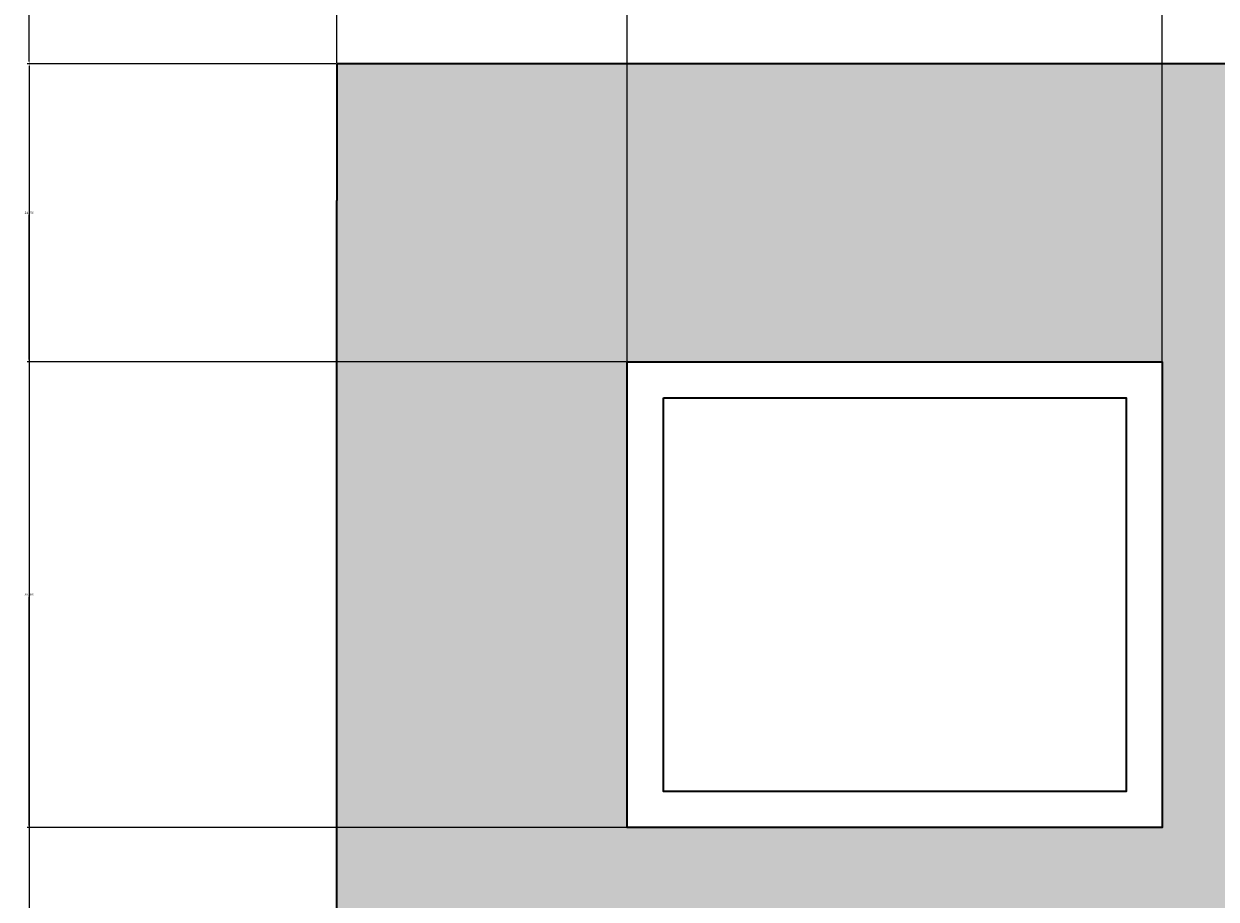
# Model space of a CAD drawing. Units: inches. Extents: x 93 to 565, y 123 to 656.
# Tile 6 of 18: x 93 to 192, y 450 to 522. Entities that reach past the tile are written whole.
import ezdxf

# ---------------------------------------------------------------- set-up
doc = ezdxf.new("R2010")
doc.units = ezdxf.units.IN
doc.header["$MEASUREMENT"] = 0
for name, color, linetype, lineweight in [('A-ANNO-DIMS', 2, 'Continuous', 18), ('A-ELEV', 7, 'Continuous', 35), ('A-WALL-PATT', 8, 'Continuous', 13)]:
    doc.layers.add(name, color=color, linetype=linetype, lineweight=lineweight)
doc.styles.get("Standard").update_dxf_attribs({"font": 'arial.ttf'})
doc.dimstyles.get("Standard").update_dxf_attribs({"dimtxt": 0.18, "dimasz": 0.18, "dimexe": 0.18, "dimexo": 0.0625, "dimgap": 0.09, "dimtad": 0, "dimtih": 1, "dimtoh": 1, "dimdec": 4, "dimzin": 0, "dimdsep": 46, "dimtxsty": 'Standard', "dimcen": 0.09, "dimadec": 0, "dimazin": 0, "dimtfac": 1, "dimtdec": 4, "dimtofl": 0, "dimtmove": 0, "dimatfit": 3, "dimfxl": 1, "dimtolj": 1, "dimtzin": 0, "dimarcsym": 0})

# ---------------------------------------------------------------- blocks, each defined once
blk = doc.blocks.new('*D26')
at = {"layer": 'A-ANNO-DIMS', "color": 0, "lineweight": -2, "transparency": 16777216}
for p, q in [((119.079, 519.162), (119.079, 656.135)), ((119.259, 655.955), (328.787, 655.955)), ((538.899, 655.955), (329.372, 655.955)), ((539.079, 630.467), (539.079, 656.135))]:
    blk.add_line(p, q, dxfattribs=at)
at = {"layer": 'A-ANNO-DIMS', "color": 0, "transparency": 16777216}
for points in [[(119.259, 655.985), (119.259, 655.925), (119.079, 655.955)], [(538.899, 655.985), (538.899, 655.925), (539.079, 655.955)]]:
    blk.add_solid(points, dxfattribs=at)
at = {"layer": 'Defpoints', "color": 0, "transparency": 16777216}
for p in [(539.079, 655.955), (539.079, 630.405), (119.079, 519.1)]:
    blk.add_point(p, dxfattribs=at)
at = {"layer": 'A-ANNO-DIMS', "color": 0, "transparency": 16777216, "insert": (329.079, 655.955), "char_height": 0.18, "attachment_point": 5}
blk.add_mtext('\\A1;420', dxfattribs=at)
blk = doc.blocks.new('*D27')
at = {"layer": 'A-ANNO-DIMS', "color": 0, "lineweight": -2, "transparency": 16777216}
for p, q in [((210.544, 519.037), (210.544, 134.002)), ((119.079, 159.67), (119.079, 134.002)), ((119.259, 134.182), (164.418, 134.182)), ((210.364, 134.182), (165.205, 134.182))]:
    blk.add_line(p, q, dxfattribs=at)
at = {"layer": 'A-ANNO-DIMS', "color": 0, "transparency": 16777216}
for points in [[(119.259, 134.212), (119.259, 134.152), (119.079, 134.182)], [(210.364, 134.212), (210.364, 134.152), (210.544, 134.182)]]:
    blk.add_solid(points, dxfattribs=at)
at = {"layer": 'Defpoints', "color": 0, "transparency": 16777216}
for p in [(210.544, 519.1), (119.079, 159.732), (210.544, 134.182)]:
    blk.add_point(p, dxfattribs=at)
at = {"layer": 'A-ANNO-DIMS', "color": 0, "transparency": 16777216, "insert": (164.812, 134.182), "char_height": 0.18, "attachment_point": 5}
blk.add_mtext('\\A1;91.46', dxfattribs=at)
blk = doc.blocks.new('*D31')
at = {"layer": 'A-ANNO-DIMS', "color": 0, "lineweight": -2, "transparency": 16777216}
for p, q in [((417.872, 630.405), (564.809, 630.405)), ((564.629, 630.225), (564.629, 395.25)), ((564.629, 159.912), (564.629, 394.887)), ((119.142, 159.732), (564.809, 159.732))]:
    blk.add_line(p, q, dxfattribs=at)
at = {"layer": 'A-ANNO-DIMS', "color": 0, "transparency": 16777216}
for points in [[(564.599, 630.225), (564.659, 630.225), (564.629, 630.405)], [(564.599, 159.912), (564.659, 159.912), (564.629, 159.732)]]:
    blk.add_solid(points, dxfattribs=at)
at = {"layer": 'Defpoints', "color": 0, "transparency": 16777216}
for p in [(417.81, 630.405), (564.629, 630.405), (119.079, 159.732)]:
    blk.add_point(p, dxfattribs=at)
at = {"layer": 'A-ANNO-DIMS', "color": 0, "transparency": 16777216, "insert": (564.629, 395.069), "char_height": 0.18, "attachment_point": 5}
blk.add_mtext('\\A1;470.7', dxfattribs=at)
blk = doc.blocks.new('*D35')
at = {"layer": 'A-ANNO-DIMS', "color": 0, "lineweight": -2, "transparency": 16777216}
for p, q in [((119.017, 519.1), (93.349, 519.1)), ((93.529, 518.92), (93.529, 441.598)), ((93.529, 363.912), (93.529, 441.234)), ((286.625, 363.732), (93.349, 363.732))]:
    blk.add_line(p, q, dxfattribs=at)
at = {"layer": 'A-ANNO-DIMS', "color": 0, "transparency": 16777216}
for points in [[(93.499, 518.92), (93.559, 518.92), (93.529, 519.1)], [(93.499, 363.912), (93.559, 363.912), (93.529, 363.732)]]:
    blk.add_solid(points, dxfattribs=at)
at = {"layer": 'Defpoints', "color": 0, "transparency": 16777216}
for p in [(93.529, 519.1), (119.079, 519.1), (286.687, 363.732)]:
    blk.add_point(p, dxfattribs=at)
at = {"layer": 'A-ANNO-DIMS', "color": 0, "transparency": 16777216, "insert": (93.529, 441.416), "char_height": 0.18, "attachment_point": 5}
blk.add_mtext('\\A1;155.37', dxfattribs=at)
blk = doc.blocks.new('*D36')
at = {"layer": 'A-ANNO-DIMS', "color": 0, "lineweight": -2, "transparency": 16777216}
for p, q in [((417.747, 594.405), (93.349, 594.405)), ((93.529, 594.225), (93.529, 556.934)), ((93.529, 519.28), (93.529, 556.57)), ((119.017, 519.1), (93.349, 519.1))]:
    blk.add_line(p, q, dxfattribs=at)
at = {"layer": 'A-ANNO-DIMS', "color": 0, "transparency": 16777216}
for points in [[(93.499, 594.225), (93.559, 594.225), (93.529, 594.405)], [(93.499, 519.28), (93.559, 519.28), (93.529, 519.1)]]:
    blk.add_solid(points, dxfattribs=at)
at = {"layer": 'Defpoints', "color": 0, "transparency": 16777216}
for p in [(93.529, 594.405), (417.81, 594.405), (119.079, 519.1)]:
    blk.add_point(p, dxfattribs=at)
at = {"layer": 'A-ANNO-DIMS', "color": 0, "transparency": 16777216, "insert": (93.529, 556.752), "char_height": 0.18, "attachment_point": 5}
blk.add_mtext('\\A1;75.3', dxfattribs=at)
blk = doc.blocks.new('*D46')
at = {"layer": 'A-ANNO-DIMS', "color": 0, "lineweight": -2, "transparency": 16777216}
for p, q in [((143.149, 455.658), (93.349, 455.658)), ((93.529, 455.478), (93.529, 443.086)), ((93.529, 430.331), (93.529, 442.722)), ((143.149, 430.151), (93.349, 430.151))]:
    blk.add_line(p, q, dxfattribs=at)
at = {"layer": 'A-ANNO-DIMS', "color": 0, "transparency": 16777216}
for points in [[(93.499, 455.478), (93.559, 455.478), (93.529, 455.658)], [(93.499, 430.331), (93.559, 430.331), (93.529, 430.151)]]:
    blk.add_solid(points, dxfattribs=at)
at = {"layer": 'Defpoints', "color": 0, "transparency": 16777216}
for p in [(93.529, 455.658), (143.212, 455.658), (143.212, 430.151)]:
    blk.add_point(p, dxfattribs=at)
at = {"layer": 'A-ANNO-DIMS', "color": 0, "transparency": 16777216, "insert": (93.529, 442.904), "char_height": 0.18, "attachment_point": 5}
blk.add_mtext('\\A1;25.507', dxfattribs=at)
blk = doc.blocks.new('*D47')
at = {"layer": 'A-ANNO-DIMS', "color": 0, "lineweight": -2, "transparency": 16777216}
for p, q in [((143.149, 494.343), (93.349, 494.343)), ((93.529, 494.163), (93.529, 475.183)), ((93.529, 455.838), (93.529, 474.819)), ((143.149, 455.658), (93.349, 455.658))]:
    blk.add_line(p, q, dxfattribs=at)
at = {"layer": 'A-ANNO-DIMS', "color": 0, "transparency": 16777216}
for points in [[(93.499, 494.163), (93.559, 494.163), (93.529, 494.343)], [(93.499, 455.838), (93.559, 455.838), (93.529, 455.658)]]:
    blk.add_solid(points, dxfattribs=at)
at = {"layer": 'Defpoints', "color": 0, "transparency": 16777216}
for p in [(93.529, 494.343), (143.212, 494.343), (143.212, 455.658)]:
    blk.add_point(p, dxfattribs=at)
at = {"layer": 'A-ANNO-DIMS', "color": 0, "transparency": 16777216, "insert": (93.529, 475.001), "char_height": 0.18, "attachment_point": 5}
blk.add_mtext('\\A1;38.685', dxfattribs=at)
blk = doc.blocks.new('*D48')
at = {"layer": 'A-ANNO-DIMS', "color": 0, "lineweight": -2, "transparency": 16777216}
for p, q in [((119.017, 519.1), (93.349, 519.1)), ((93.529, 518.92), (93.529, 506.904)), ((93.529, 494.523), (93.529, 506.54)), ((143.149, 494.343), (93.349, 494.343))]:
    blk.add_line(p, q, dxfattribs=at)
at = {"layer": 'A-ANNO-DIMS', "color": 0, "transparency": 16777216}
for points in [[(93.499, 518.92), (93.559, 518.92), (93.529, 519.1)], [(93.499, 494.523), (93.559, 494.523), (93.529, 494.343)]]:
    blk.add_solid(points, dxfattribs=at)
at = {"layer": 'Defpoints', "color": 0, "transparency": 16777216}
for p in [(93.529, 519.1), (119.079, 519.1), (143.212, 494.343)]:
    blk.add_point(p, dxfattribs=at)
at = {"layer": 'A-ANNO-DIMS', "color": 0, "transparency": 16777216, "insert": (93.529, 506.722), "char_height": 0.18, "attachment_point": 5}
blk.add_mtext('\\A1;24.756', dxfattribs=at)
blk = doc.blocks.new('*D49')
at = {"layer": 'A-ANNO-DIMS', "color": 0, "lineweight": -2, "transparency": 16777216}
for p, q in [((119.079, 519.162), (119.079, 656.135)), ((119.259, 655.955), (130.75, 655.955)), ((143.032, 655.955), (131.541, 655.955)), ((143.212, 494.406), (143.212, 656.135))]:
    blk.add_line(p, q, dxfattribs=at)
at = {"layer": 'A-ANNO-DIMS', "color": 0, "transparency": 16777216}
for points in [[(119.259, 655.985), (119.259, 655.925), (119.079, 655.955)], [(143.032, 655.985), (143.032, 655.925), (143.212, 655.955)]]:
    blk.add_solid(points, dxfattribs=at)
at = {"layer": 'Defpoints', "color": 0, "transparency": 16777216}
for p in [(143.212, 655.955), (119.079, 519.1), (143.212, 494.343)]:
    blk.add_point(p, dxfattribs=at)
at = {"layer": 'A-ANNO-DIMS', "color": 0, "transparency": 16777216, "insert": (131.146, 655.955), "char_height": 0.18, "attachment_point": 5}
blk.add_mtext('\\A1;24.13', dxfattribs=at)
blk = doc.blocks.new('*D50')
at = {"layer": 'A-ANNO-DIMS', "color": 0, "lineweight": -2, "transparency": 16777216}
for p, q in [((143.212, 494.406), (143.212, 656.135)), ((143.392, 655.955), (165.033, 655.955)), ((187.468, 655.955), (165.827, 655.955)), ((187.648, 494.406), (187.648, 656.135))]:
    blk.add_line(p, q, dxfattribs=at)
at = {"layer": 'A-ANNO-DIMS', "color": 0, "transparency": 16777216}
for points in [[(143.392, 655.985), (143.392, 655.925), (143.212, 655.955)], [(187.468, 655.985), (187.468, 655.925), (187.648, 655.955)]]:
    blk.add_solid(points, dxfattribs=at)
at = {"layer": 'Defpoints', "color": 0, "transparency": 16777216}
for p in [(187.648, 655.955), (143.212, 494.343), (187.648, 494.343)]:
    blk.add_point(p, dxfattribs=at)
at = {"layer": 'A-ANNO-DIMS', "color": 0, "transparency": 16777216, "insert": (165.43, 655.955), "char_height": 0.18, "attachment_point": 5}
blk.add_mtext('\\A1;44.44', dxfattribs=at)
blk = doc.blocks.new('*D105')
at = {"layer": 'A-ANNO-DIMS', "color": 0, "lineweight": -2, "transparency": 16777216}
for p, q in [((119.079, 519.162), (119.079, 656.135)), ((119.259, 655.955), (328.542, 655.955)), ((538.899, 655.955), (329.616, 655.955)), ((539.079, 630.467), (539.079, 656.135))]:
    blk.add_line(p, q, dxfattribs=at)
at = {"layer": 'A-ANNO-DIMS', "color": 0, "transparency": 16777216}
for points in [[(119.259, 655.985), (119.259, 655.925), (119.079, 655.955)], [(538.899, 655.985), (538.899, 655.925), (539.079, 655.955)]]:
    blk.add_solid(points, dxfattribs=at)
at = {"layer": 'Defpoints', "color": 0, "transparency": 16777216}
for p in [(539.079, 655.955), (539.079, 630.405), (119.079, 519.1)]:
    blk.add_point(p, dxfattribs=at)
at = {"layer": 'A-ANNO-DIMS', "color": 0, "transparency": 16777216, "insert": (329.079, 655.955), "char_height": 0.18, "attachment_point": 5}
blk.add_mtext('\\A1;420.000', dxfattribs=at)
blk = doc.blocks.new('*D106')
at = {"layer": 'A-ANNO-DIMS', "color": 0, "lineweight": -2, "transparency": 16777216}
for p, q in [((210.544, 519.037), (210.544, 134.002)), ((119.079, 159.67), (119.079, 134.002)), ((119.259, 134.182), (164.348, 134.182)), ((210.364, 134.182), (165.276, 134.182))]:
    blk.add_line(p, q, dxfattribs=at)
at = {"layer": 'A-ANNO-DIMS', "color": 0, "transparency": 16777216}
for points in [[(119.259, 134.212), (119.259, 134.152), (119.079, 134.182)], [(210.364, 134.212), (210.364, 134.152), (210.544, 134.182)]]:
    blk.add_solid(points, dxfattribs=at)
at = {"layer": 'Defpoints', "color": 0, "transparency": 16777216}
for p in [(210.544, 519.1), (119.079, 159.732), (210.544, 134.182)]:
    blk.add_point(p, dxfattribs=at)
at = {"layer": 'A-ANNO-DIMS', "color": 0, "transparency": 16777216, "insert": (164.812, 134.182), "char_height": 0.18, "attachment_point": 5}
blk.add_mtext('\\A1;91.465', dxfattribs=at)
blk = doc.blocks.new('*D110')
at = {"layer": 'A-ANNO-DIMS', "color": 0, "lineweight": -2, "transparency": 16777216}
for p, q in [((417.872, 630.405), (564.809, 630.405)), ((564.629, 630.225), (564.629, 395.25)), ((564.629, 159.912), (564.629, 394.887)), ((119.142, 159.732), (564.809, 159.732))]:
    blk.add_line(p, q, dxfattribs=at)
at = {"layer": 'A-ANNO-DIMS', "color": 0, "transparency": 16777216}
for points in [[(564.599, 630.225), (564.659, 630.225), (564.629, 630.405)], [(564.599, 159.912), (564.659, 159.912), (564.629, 159.732)]]:
    blk.add_solid(points, dxfattribs=at)
at = {"layer": 'Defpoints', "color": 0, "transparency": 16777216}
for p in [(417.81, 630.405), (564.629, 630.405), (119.079, 159.732)]:
    blk.add_point(p, dxfattribs=at)
at = {"layer": 'A-ANNO-DIMS', "color": 0, "transparency": 16777216, "insert": (564.629, 395.069), "char_height": 0.18, "attachment_point": 5}
blk.add_mtext('\\A1;470.673', dxfattribs=at)
blk = doc.blocks.new('*D114')
at = {"layer": 'A-ANNO-DIMS', "color": 0, "lineweight": -2, "transparency": 16777216}
for p, q in [((119.017, 519.1), (93.349, 519.1)), ((93.529, 518.92), (93.529, 441.598)), ((93.529, 363.912), (93.529, 441.234)), ((286.625, 363.732), (93.349, 363.732))]:
    blk.add_line(p, q, dxfattribs=at)
at = {"layer": 'A-ANNO-DIMS', "color": 0, "transparency": 16777216}
for points in [[(93.499, 518.92), (93.559, 518.92), (93.529, 519.1)], [(93.499, 363.912), (93.559, 363.912), (93.529, 363.732)]]:
    blk.add_solid(points, dxfattribs=at)
at = {"layer": 'Defpoints', "color": 0, "transparency": 16777216}
for p in [(93.529, 519.1), (119.079, 519.1), (286.687, 363.732)]:
    blk.add_point(p, dxfattribs=at)
at = {"layer": 'A-ANNO-DIMS', "color": 0, "transparency": 16777216, "insert": (93.529, 441.416), "char_height": 0.18, "attachment_point": 5}
blk.add_mtext('\\A1;155.368', dxfattribs=at)
blk = doc.blocks.new('*D115')
at = {"layer": 'A-ANNO-DIMS', "color": 0, "lineweight": -2, "transparency": 16777216}
for p, q in [((417.747, 594.405), (93.349, 594.405)), ((93.529, 594.225), (93.529, 556.934)), ((93.529, 519.28), (93.529, 556.57)), ((119.017, 519.1), (93.349, 519.1))]:
    blk.add_line(p, q, dxfattribs=at)
at = {"layer": 'A-ANNO-DIMS', "color": 0, "transparency": 16777216}
for points in [[(93.499, 594.225), (93.559, 594.225), (93.529, 594.405)], [(93.499, 519.28), (93.559, 519.28), (93.529, 519.1)]]:
    blk.add_solid(points, dxfattribs=at)
at = {"layer": 'Defpoints', "color": 0, "transparency": 16777216}
for p in [(93.529, 594.405), (417.81, 594.405), (119.079, 519.1)]:
    blk.add_point(p, dxfattribs=at)
at = {"layer": 'A-ANNO-DIMS', "color": 0, "transparency": 16777216, "insert": (93.529, 556.752), "char_height": 0.18, "attachment_point": 5}
blk.add_mtext('\\A1;75.305', dxfattribs=at)
blk = doc.blocks.new('*D125')
at = {"layer": 'A-ANNO-DIMS', "color": 0, "lineweight": -2, "transparency": 16777216}
for p, q in [((143.149, 455.658), (93.349, 455.658)), ((93.529, 455.478), (93.529, 443.086)), ((93.529, 430.331), (93.529, 442.722)), ((143.149, 430.151), (93.349, 430.151))]:
    blk.add_line(p, q, dxfattribs=at)
at = {"layer": 'A-ANNO-DIMS', "color": 0, "transparency": 16777216}
for points in [[(93.499, 455.478), (93.559, 455.478), (93.529, 455.658)], [(93.499, 430.331), (93.559, 430.331), (93.529, 430.151)]]:
    blk.add_solid(points, dxfattribs=at)
at = {"layer": 'Defpoints', "color": 0, "transparency": 16777216}
for p in [(93.529, 455.658), (143.212, 455.658), (143.212, 430.151)]:
    blk.add_point(p, dxfattribs=at)
at = {"layer": 'A-ANNO-DIMS', "color": 0, "transparency": 16777216, "insert": (93.529, 442.904), "char_height": 0.18, "attachment_point": 5}
blk.add_mtext('\\A1;25.507', dxfattribs=at)
blk = doc.blocks.new('*D126')
at = {"layer": 'A-ANNO-DIMS', "color": 0, "lineweight": -2, "transparency": 16777216}
for p, q in [((143.149, 494.343), (93.349, 494.343)), ((93.529, 494.163), (93.529, 475.183)), ((93.529, 455.838), (93.529, 474.819)), ((143.149, 455.658), (93.349, 455.658))]:
    blk.add_line(p, q, dxfattribs=at)
at = {"layer": 'A-ANNO-DIMS', "color": 0, "transparency": 16777216}
for points in [[(93.499, 494.163), (93.559, 494.163), (93.529, 494.343)], [(93.499, 455.838), (93.559, 455.838), (93.529, 455.658)]]:
    blk.add_solid(points, dxfattribs=at)
at = {"layer": 'Defpoints', "color": 0, "transparency": 16777216}
for p in [(93.529, 494.343), (143.212, 494.343), (143.212, 455.658)]:
    blk.add_point(p, dxfattribs=at)
at = {"layer": 'A-ANNO-DIMS', "color": 0, "transparency": 16777216, "insert": (93.529, 475.001), "char_height": 0.18, "attachment_point": 5}
blk.add_mtext('\\A1;38.685', dxfattribs=at)
blk = doc.blocks.new('*D127')
at = {"layer": 'A-ANNO-DIMS', "color": 0, "lineweight": -2, "transparency": 16777216}
for p, q in [((119.017, 519.1), (93.349, 519.1)), ((93.529, 518.92), (93.529, 506.904)), ((93.529, 494.523), (93.529, 506.54)), ((143.149, 494.343), (93.349, 494.343))]:
    blk.add_line(p, q, dxfattribs=at)
at = {"layer": 'A-ANNO-DIMS', "color": 0, "transparency": 16777216}
for points in [[(93.499, 518.92), (93.559, 518.92), (93.529, 519.1)], [(93.499, 494.523), (93.559, 494.523), (93.529, 494.343)]]:
    blk.add_solid(points, dxfattribs=at)
at = {"layer": 'Defpoints', "color": 0, "transparency": 16777216}
for p in [(93.529, 519.1), (119.079, 519.1), (143.212, 494.343)]:
    blk.add_point(p, dxfattribs=at)
at = {"layer": 'A-ANNO-DIMS', "color": 0, "transparency": 16777216, "insert": (93.529, 506.722), "char_height": 0.18, "attachment_point": 5}
blk.add_mtext('\\A1;24.756', dxfattribs=at)
blk = doc.blocks.new('*D128')
at = {"layer": 'A-ANNO-DIMS', "color": 0, "lineweight": -2, "transparency": 16777216}
for p, q in [((119.079, 519.162), (119.079, 656.135)), ((119.259, 655.955), (130.681, 655.955)), ((143.032, 655.955), (131.61, 655.955)), ((143.212, 494.406), (143.212, 656.135))]:
    blk.add_line(p, q, dxfattribs=at)
at = {"layer": 'A-ANNO-DIMS', "color": 0, "transparency": 16777216}
for points in [[(119.259, 655.985), (119.259, 655.925), (119.079, 655.955)], [(143.032, 655.985), (143.032, 655.925), (143.212, 655.955)]]:
    blk.add_solid(points, dxfattribs=at)
at = {"layer": 'Defpoints', "color": 0, "transparency": 16777216}
for p in [(143.212, 655.955), (119.079, 519.1), (143.212, 494.343)]:
    blk.add_point(p, dxfattribs=at)
at = {"layer": 'A-ANNO-DIMS', "color": 0, "transparency": 16777216, "insert": (131.146, 655.955), "char_height": 0.18, "attachment_point": 5}
blk.add_mtext('\\A1;24.132', dxfattribs=at)
blk = doc.blocks.new('*D129')
at = {"layer": 'A-ANNO-DIMS', "color": 0, "lineweight": -2, "transparency": 16777216}
for p, q in [((143.212, 494.406), (143.212, 656.135)), ((143.392, 655.955), (164.963, 655.955)), ((187.468, 655.955), (165.897, 655.955)), ((187.648, 494.406), (187.648, 656.135))]:
    blk.add_line(p, q, dxfattribs=at)
at = {"layer": 'A-ANNO-DIMS', "color": 0, "transparency": 16777216}
for points in [[(143.392, 655.985), (143.392, 655.925), (143.212, 655.955)], [(187.468, 655.985), (187.468, 655.925), (187.648, 655.955)]]:
    blk.add_solid(points, dxfattribs=at)
at = {"layer": 'Defpoints', "color": 0, "transparency": 16777216}
for p in [(187.648, 655.955), (143.212, 494.343), (187.648, 494.343)]:
    blk.add_point(p, dxfattribs=at)
at = {"layer": 'A-ANNO-DIMS', "color": 0, "transparency": 16777216, "insert": (165.43, 655.955), "char_height": 0.18, "attachment_point": 5}
blk.add_mtext('\\A1;44.436', dxfattribs=at)

msp = doc.modelspace()

# ---------------------------------------------------------------- hatches: boundary and pattern name
at = {"layer": 'A-WALL-PATT'}
h = msp.add_hatch(dxfattribs=at)
h.set_pattern_fill('STARS', color=256, scale=21)
h.paths.add_polyline_path([(210.5443, 507.7323), (210.5443, 519.0999), (119.0794, 519.0999), (119.0794, 507.7323), (119.0794, 183.7323), (210.5443, 183.7323)])
h.paths.add_polyline_path([(187.648, 430.1508), (187.648, 391.4653), (143.2118, 391.4653), (143.2118, 430.1508)], flags=16)
h.paths.add_polyline_path([(187.648, 455.6579), (143.2118, 455.6579), (143.2118, 494.3434), (187.648, 494.3434)], flags=16)
h.paths.add_polyline_path([(184.648, 427.1508), (184.648, 394.4653), (146.2118, 394.4653), (146.2118, 427.1508)], flags=0)
h.paths.add_polyline_path([(184.648, 458.6579), (146.2118, 458.6579), (146.2118, 491.3434), (184.648, 491.3434)], flags=0)
h.paths.add_polyline_path([(187.648, 363.1705), (187.648, 324.485), (143.2118, 324.485), (143.2118, 363.1705)], flags=16)
h.paths.add_polyline_path([(184.648, 360.1705), (184.648, 327.485), (146.2118, 327.485), (146.2118, 360.1705)], flags=0)
h.paths.add_polyline_path([(187.648, 300.3249), (187.648, 261.6394), (143.2118, 261.6394), (143.2118, 300.3249)], flags=16)
h.paths.add_polyline_path([(184.648, 297.3249), (184.648, 264.6394), (146.2118, 264.6394), (146.2118, 297.3249)], flags=0)
h.paths.add_polyline_path([(187.648, 243.6441), (187.648, 204.9587), (143.2118, 204.9587), (143.2118, 243.6441)], flags=16)
h.paths.add_polyline_path([(184.648, 240.6441), (184.648, 207.9587), (146.2118, 207.9587), (146.2118, 240.6441)], flags=0)

# ---------------------------------------------------------------- linework, layer by layer
at = {"layer": 'A-ELEV'}
for p, q in [((210.5443, 519.0999), (119.0794, 519.0999)), ((119.0794, 519.0999), (119.0794, 507.7323)), ((119.0794, 183.7323), (119.0794, 507.7323))]:
    msp.add_line(p, q, dxfattribs=at)
for points in [[(143.2118, 494.3434), (187.648, 494.3434), (187.648, 455.6579), (143.2118, 455.6579)], [(146.2118, 491.3434), (184.648, 491.3434), (184.648, 458.6579), (146.2118, 458.6579)]]:
    msp.add_lwpolyline(points, close=True, dxfattribs=at)

# ---------------------------------------------------------------- dimensions: what is measured, and where the dimension line sits
at = {"layer": 'A-ANNO-DIMS'}
for base, p1, p2, override, picture, middle in [((539.0794, 655.9548), (119.0794, 519.0999), (539.0794, 630.4048), {"dimdec": 0, "dimlfac": 1, "dimrnd": 0, "dimzin": 0, "dimdsep": 46, "dimlunit": 2}, '*D26', (329.0794, 655.9548)), ((143.2118, 655.9548), (119.0794, 519.0999), (143.2118, 494.3434), {"dimdec": 2, "dimlfac": 1, "dimrnd": 0, "dimzin": 0, "dimdsep": 46, "dimlunit": 2}, '*D49', (131.1456, 655.9548)), ((539.0794, 655.9548), (119.0794, 519.0999), (539.0794, 630.4048), {"dimdec": 3, "dimlfac": 1, "dimrnd": 0, "dimzin": 0, "dimdsep": 46, "dimlunit": 2}, '*D105', (329.0794, 655.9548)), ((143.2118, 655.9548), (119.0794, 519.0999), (143.2118, 494.3434), {"dimdec": 3, "dimlfac": 1, "dimrnd": 0, "dimzin": 0, "dimdsep": 46, "dimlunit": 2}, '*D128', (131.1456, 655.9548)), ((187.648, 655.9548), (143.2118, 494.3434), (187.648, 494.3434), {"dimdec": 2, "dimlfac": 1, "dimrnd": 0, "dimzin": 0, "dimdsep": 46, "dimlunit": 2}, '*D50', (165.4299, 655.9548)), ((187.648, 655.9548), (143.2118, 494.3434), (187.648, 494.3434), {"dimdec": 3, "dimlfac": 1, "dimrnd": 0, "dimzin": 0, "dimdsep": 46, "dimlunit": 2}, '*D129', (165.4299, 655.9548)), ((210.5443, 134.1823), (119.0794, 159.7323), (210.5443, 519.0999), {"dimdec": 2, "dimlfac": 1, "dimrnd": 0, "dimzin": 0, "dimdsep": 46, "dimlunit": 2}, '*D27', (164.8118, 134.1823)), ((210.5443, 134.1823), (119.0794, 159.7323), (210.5443, 519.0999), {"dimdec": 3, "dimlfac": 1, "dimrnd": 0, "dimzin": 0, "dimdsep": 46, "dimlunit": 2}, '*D106', (164.8118, 134.1823))]:
    dim = msp.add_linear_dim(base=base, p1=p1, p2=p2, dimstyle='Standard', override=override, dxfattribs=at)
    dim.commit()
    dim.dimension.update_dxf_attribs({"geometry": picture, "text_midpoint": middle})
for base, p1, p2, override, picture, middle in [((564.6294, 630.4048), (119.0794, 159.7323), (417.8097, 630.4048), {"dimdec": 1, "dimlfac": 1, "dimrnd": 0, "dimzin": 0, "dimdsep": 46, "dimlunit": 2}, '*D31', (564.6294, 395.0685)), ((564.62936, 630.40478), (119.07936, 159.73225), (417.80971, 630.40477), {"dimdec": 3, "dimlfac": 1, "dimrnd": 0, "dimzin": 0, "dimdsep": 46, "dimlunit": 2}, '*D110', (564.62936, 395.06851)), ((93.5294, 594.4048), (119.0794, 519.0999), (417.8097, 594.4048), {"dimdec": 3, "dimlfac": 1, "dimrnd": 0, "dimzin": 0, "dimdsep": 46, "dimlunit": 2}, '*D115', (93.5294, 556.7523)), ((93.5294, 594.4048), (119.0794, 519.0999), (417.8097, 594.4048), {"dimdec": 1, "dimlfac": 1, "dimrnd": 0, "dimzin": 0, "dimdsep": 46, "dimlunit": 2}, '*D36', (93.5294, 556.7523)), ((93.5294, 519.0999), (286.6874, 363.7323), (119.0794, 519.0999), {"dimdec": 3, "dimlfac": 1, "dimrnd": 0, "dimzin": 0, "dimdsep": 46, "dimlunit": 2}, '*D114', (93.5294, 441.4161)), ((93.5294, 519.0999), (286.6874, 363.7323), (119.0794, 519.0999), {"dimdec": 2, "dimlfac": 1, "dimrnd": 0, "dimzin": 0, "dimdsep": 46, "dimlunit": 2}, '*D35', (93.5294, 441.4161)), ((93.52936, 519.09987), (143.21177, 494.34341), (119.07936, 519.09987), {"dimdec": 3, "dimlfac": 1, "dimrnd": 0, "dimzin": 0, "dimdsep": 46, "dimlunit": 2}, '*D48', (93.52936, 506.72164)), ((93.52936, 519.09987), (143.21177, 494.34341), (119.07936, 519.09987), {"dimdec": 3, "dimlfac": 1, "dimrnd": 0, "dimzin": 0, "dimdsep": 46, "dimlunit": 2}, '*D127', (93.52936, 506.72164)), ((93.52936, 494.34341), (143.21177, 455.65794), (143.21177, 494.34341), {"dimdec": 3, "dimlfac": 1, "dimrnd": 0, "dimzin": 0, "dimdsep": 46, "dimlunit": 2}, '*D47', (93.52936, 475.00068)), ((93.52936, 494.34341), (143.21177, 455.65794), (143.21177, 494.34341), {"dimdec": 3, "dimlfac": 1, "dimrnd": 0, "dimzin": 0, "dimdsep": 46, "dimlunit": 2}, '*D126', (93.52936, 475.00068)), ((93.5294, 455.6579), (143.2118, 430.1508), (143.2118, 455.6579), {"dimdec": 3, "dimlfac": 1, "dimrnd": 0, "dimzin": 0, "dimdsep": 46, "dimlunit": 2}, '*D46', (93.5294, 442.9043)), ((93.5294, 455.6579), (143.2118, 430.1508), (143.2118, 455.6579), {"dimdec": 3, "dimlfac": 1, "dimrnd": 0, "dimzin": 0, "dimdsep": 46, "dimlunit": 2}, '*D125', (93.5294, 442.9043))]:
    dim = msp.add_linear_dim(base=base, p1=p1, p2=p2, angle=90, dimstyle='Standard', override=override, dxfattribs=at)
    dim.commit()
    dim.dimension.update_dxf_attribs({"geometry": picture, "text_midpoint": middle})

doc.saveas('drawing.dxf')
